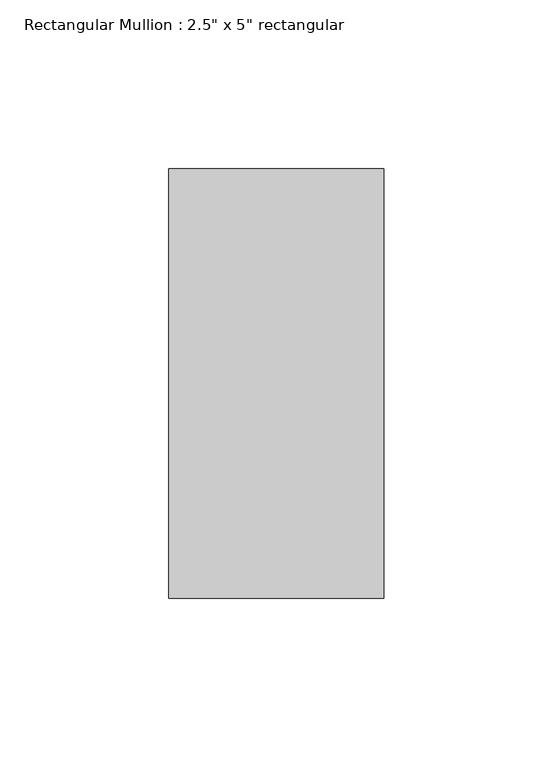
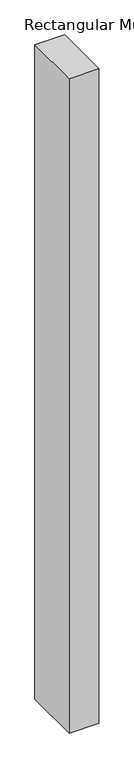
"""IFC4 building model written with IfcOpenShell, lengths in millimetres: member geometry."""

from ifc_helpers import new_model, si_unit, frame, origin, place, context, project, spatial, polyline, outline, extrude, source, transform, mapped, element, save


def member_7a8c6f17(model_context):
    return source(origin(), model_context, "Body", "SweptSolid", [
        extrude(outline(polyline([(31.75, 63.5), (31.75, -63.5), (-31.75, -63.5), (-31.75, 63.5), (31.75, 63.5)])), frame((0.0, 0.0, -1478.7314865), z_axis=(0.0, 0.0, 1.0), x_axis=(1.0, 0.0, 0.0)), (0.0, 0.0, 1.0), 1478.7314865),
    ])


if __name__ == "__main__":
    model = new_model("IFC4")
    model_context = context("Model", 3, world=origin())
    ifc_project = project(units=[si_unit("LENGTHUNIT", "METRE", prefix="MILLI")], contexts=[model_context])
    site = spatial("IfcSite", under=ifc_project)
    building = spatial("IfcBuilding", under=site)
    placement = place(None, origin())
    member_shape = member_7a8c6f17(model_context)
    element("IfcMember", 1, ObjectType="Rectangular Mullion : 2.5\" x 5\" rectangular", at=placement, inside=building, context=model_context, shape_type="MappedRepresentation", body=[
        mapped(member_shape, transform((0.0, 0.0, 0.0), x_axis=(1.0, 0.0, 0.0), y_axis=(0.0, 1.0, 0.0), z_axis=(0.0, 0.0, 1.0))),
    ])
    save(model, "model.ifc")

# Revit data of these elements
# Type "Rectangular Mullion : 2.5\" x 5\" rectangular"
#   built-in parameter 1007304 = 0.416667 (stored number, unit not read)
#   built-in parameter 1007301 = 0.104167 (stored number, unit not read)
#   built-in parameter 1007300 = 0.104167 (stored number, unit not read)
# Element 1 (IfcMember, "Rectangular Mullion : 2.5\" x 5\" rectangular")
#   Materials on its faces: "Aluminum"
# Materials
#   "Aluminum": class "Metal", colour RGB 247 247 247, transparency 0, Description = "Aluminum 6061", Cost = 0
